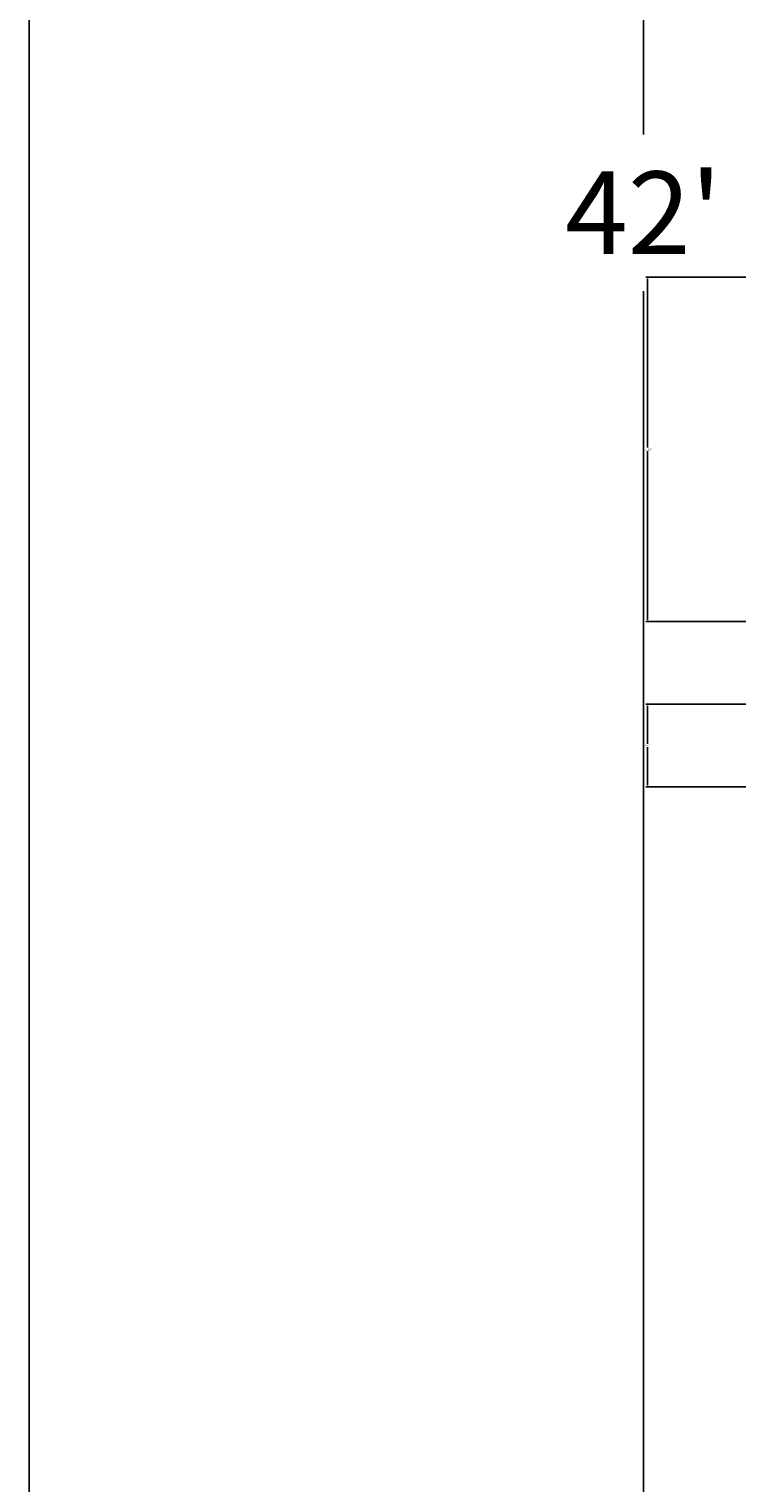
# Model space of a CAD drawing. Units: inches. Extents: x 311 to 815, y -527 to 136.
# Tile 5 of 21: x 311 to 388, y -368 to -210. Entities that reach past the tile are written whole.
import ezdxf

# ---------------------------------------------------------------- set-up
doc = ezdxf.new("R2010")
doc.units = ezdxf.units.IN
doc.header["$MEASUREMENT"] = 0
doc.layers.add('A-ANNO-DIMS', color=1, linetype='Continuous', lineweight=18)
doc.layers.add('A-ANNO-TTLB', color=1, linetype='Continuous', lineweight=25)
doc.styles.get("Standard").update_dxf_attribs({"font": 'arial.ttf'})
doc.dimstyles.get("Standard").update_dxf_attribs({"dimtxt": 0.18, "dimasz": 0.18, "dimexe": 0.18, "dimexo": 0.0625, "dimgap": 0.09, "dimtad": 0, "dimtih": 1, "dimtoh": 1, "dimdec": 1, "dimzin": 0, "dimdsep": 46, "dimlunit": 4, "dimtxsty": 'Standard', "dimcen": 0.09, "dimadec": 0, "dimazin": 0, "dimtfac": 1, "dimtdec": 1, "dimtofl": 0, "dimtmove": 0, "dimatfit": 3, "dimfxl": 1, "dimtolj": 1, "dimtzin": 0, "dimarcsym": 0})

# ---------------------------------------------------------------- blocks, each defined once
blk = doc.blocks.new('_ArchTick')
at = {"color": 0, "linetype": 'ByBlock', "const_width": 0.15}
blk.add_lwpolyline([(-0.5, -0.5), (0.5, 0.5)], dxfattribs=at)
blk = doc.blocks.new('_Oblique')
at = {"color": 0, "linetype": 'ByBlock', "lineweight": -2}
blk.add_line((-0.5, -0.5), (0.5, 0.5), dxfattribs=at)
blk = doc.blocks.new('*D3')
at = {"layer": 'A-ANNO-DIMS', "color": 0, "lineweight": -2, "transparency": 16777216}
for p, q in [((377.54, 21.87), (377.54, -221.61)), ((377.54, -482.13), (377.54, -238.65))]:
    blk.add_line(p, q, dxfattribs=at)
at = {"layer": 'Defpoints', "color": 0, "transparency": 16777216}
for p in [(410.32, 21.87), (377.54, -482.13), (410.32, -482.13)]:
    blk.add_point(p, dxfattribs=at)
at = {"layer": 'A-ANNO-DIMS', "color": 0, "lineweight": -2, "transparency": 16777216, "xscale": 9, "yscale": 9, "zscale": 9}
for name, p, rotation in [('_ArchTick', (377.54, 21.87), 90), ('_Oblique', (377.54, -482.13), 270)]:
    blk.add_blockref(name, p, dxfattribs=dict(at, rotation=rotation))
at = {"layer": 'A-ANNO-DIMS', "color": 0, "transparency": 16777216, "insert": (377.54, -230.13), "char_height": 9, "attachment_point": 5}
blk.add_mtext("\\A1;42'", dxfattribs=at)
blk = doc.blocks.new('*D33')
at = {"layer": 'A-ANNO-DIMS', "color": 0, "lineweight": -2, "transparency": 16777216}
for p, q in [((609.26, -237.13), (377.79, -237.13)), ((377.97, -237.31), (377.97, -255.69)), ((377.97, -274.45), (377.97, -256.06)), ((609.26, -274.63), (377.79, -274.63))]:
    blk.add_line(p, q, dxfattribs=at)
at = {"layer": 'A-ANNO-DIMS', "color": 0, "transparency": 16777216}
for points in [[(377.94, -237.31), (378, -237.31), (377.97, -237.13)], [(377.94, -274.45), (378, -274.45), (377.97, -274.63)]]:
    blk.add_solid(points, dxfattribs=at)
at = {"layer": 'Defpoints', "color": 0, "transparency": 16777216}
for p in [(609.32, -237.13), (377.97, -274.63), (609.32, -274.63)]:
    blk.add_point(p, dxfattribs=at)
at = {"layer": 'A-ANNO-DIMS', "color": 0, "transparency": 16777216, "insert": (377.97, -255.88), "char_height": 0.18, "attachment_point": 5}
blk.add_mtext('\\A1;3\'-1 1/2"', dxfattribs=at)
blk = doc.blocks.new('*D36')
at = {"layer": 'A-ANNO-DIMS', "color": 0, "lineweight": -2, "transparency": 16777216}
for p, q in [((665.26, -283.63), (377.79, -283.63)), ((377.97, -283.81), (377.97, -287.95)), ((377.97, -292.45), (377.97, -288.31)), ((665.26, -292.63), (377.79, -292.63))]:
    blk.add_line(p, q, dxfattribs=at)
at = {"layer": 'A-ANNO-DIMS', "color": 0, "transparency": 16777216}
for points in [[(377.94, -283.81), (378, -283.81), (377.97, -283.63)], [(377.94, -292.45), (378, -292.45), (377.97, -292.63)]]:
    blk.add_solid(points, dxfattribs=at)
at = {"layer": 'Defpoints', "color": 0, "transparency": 16777216}
for p in [(665.32, -283.63), (377.97, -292.63), (665.32, -292.63)]:
    blk.add_point(p, dxfattribs=at)
at = {"layer": 'A-ANNO-DIMS', "color": 0, "transparency": 16777216, "insert": (377.97, -288.13), "char_height": 0.18, "attachment_point": 5}
blk.add_mtext('\\A1;0\'-9"', dxfattribs=at)

msp = doc.modelspace()

# ---------------------------------------------------------------- linework, layer by layer
at = {"layer": 'A-ANNO-TTLB'}
msp.add_lwpolyline([(310.67, 136.01), (815.43, 136.01), (815.43, -506.97), (310.67, -506.97)], close=True, dxfattribs=at)

# ---------------------------------------------------------------- dimensions: what is measured, and where the dimension line sits
at = {"layer": 'A-ANNO-DIMS'}
for base, p1, p2, override, picture, middle in [((377.54, -482.13), (410.32, 21.87), (410.32, -482.13), {"dimtxt": 9, "dimasz": 9, "dimgap": 4, "dimblk1": 'ArchTick', "dimblk2": 'Oblique', "dimsah": 1, "dimse1": 1, "dimse2": 1, "dimclrd": 0, "dimclre": 0, "dimclrt": 0}, '*D3', (377.54, -230.13)), ((377.97, -274.63), (609.32, -237.13), (609.32, -274.63), {"dimdec": 1, "dimlfac": 1, "dimrnd": 0, "dimzin": 1, "dimdsep": 46, "dimlunit": 4, "dimfrac": 2}, '*D33', (377.97, -255.88)), ((377.97, -292.63), (665.32, -283.63), (665.32, -292.63), {"dimdec": 1, "dimlfac": 1, "dimrnd": 0, "dimzin": 1, "dimdsep": 46, "dimlunit": 4, "dimfrac": 2}, '*D36', (377.97, -288.13))]:
    dim = msp.add_linear_dim(base=base, p1=p1, p2=p2, angle=90, dimstyle='Standard', override=override, dxfattribs=at)
    dim.commit()
    dim.dimension.update_dxf_attribs({"geometry": picture, "text_midpoint": middle})

doc.saveas('drawing.dxf')
